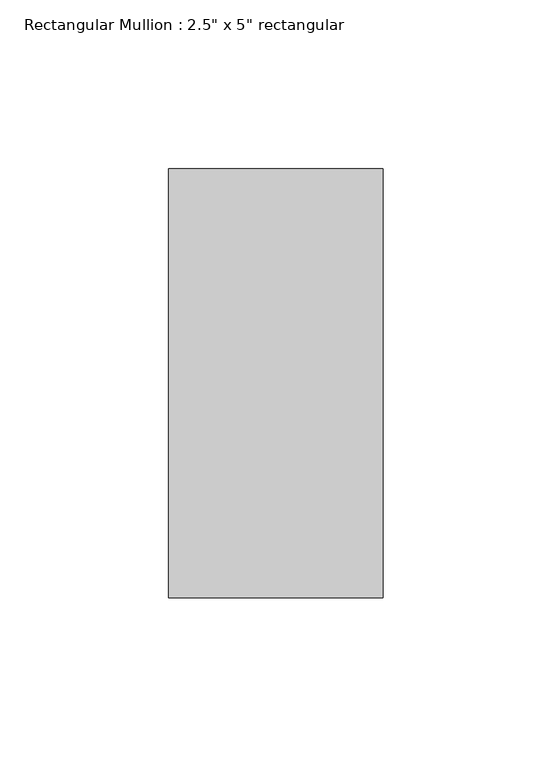
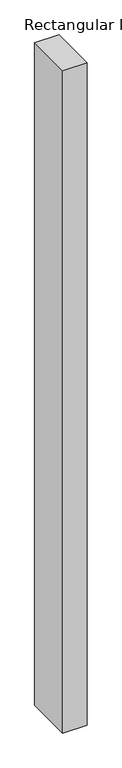
"""IFC4 building model written with IfcOpenShell, lengths in millimetres: member geometry."""

from ifc_helpers import new_model, si_unit, frame, origin, place, context, project, spatial, polyline, outline, extrude, source, transform, mapped, element, save


def member_75351bdb(model_context):
    return source(origin(), model_context, "Body", "SweptSolid", [
        extrude(outline(polyline([(0.0, 63.5), (0.0, -63.5), (-63.5, -63.5), (-63.5, 63.5), (0.0, 63.5)])), frame((0.0, 0.0, -1835.15), z_axis=(0.0, 0.0, 1.0), x_axis=(1.0, 0.0, 0.0)), (0.0, 0.0, 1.0), 1835.15),
    ])


if __name__ == "__main__":
    model = new_model("IFC4")
    model_context = context("Model", 3, world=origin())
    ifc_project = project(units=[si_unit("LENGTHUNIT", "METRE", prefix="MILLI")], contexts=[model_context])
    site = spatial("IfcSite", under=ifc_project)
    building = spatial("IfcBuilding", under=site)
    placement = place(None, origin())
    member_shape = member_75351bdb(model_context)
    element("IfcMember", 1, ObjectType="Rectangular Mullion : 2.5\" x 5\" rectangular", at=placement, inside=building, context=model_context, shape_type="MappedRepresentation", body=[
        mapped(member_shape, transform((0.0, 0.0, 0.0), x_axis=(1.0, 0.0, 0.0), y_axis=(0.0, 1.0, 0.0), z_axis=(0.0, 0.0, 1.0))),
    ])
    save(model, "model.ifc")

# Revit data of these elements
# Type "Rectangular Mullion : 2.5\" x 5\" rectangular"
#   built-in parameter 1007304 = 0.416667 (stored number, unit not read)
#   built-in parameter 1007301 = 0.104167 (stored number, unit not read)
#   built-in parameter 1007300 = 0.104167 (stored number, unit not read)
# Element 1 (IfcMember, "Rectangular Mullion : 2.5\" x 5\" rectangular")
#   Materials on its faces: "Aluminum"
# Materials
#   "Aluminum": class "Metal", colour RGB 247 247 247, transparency 0, Description = "Aluminum 6061", Cost = 0
